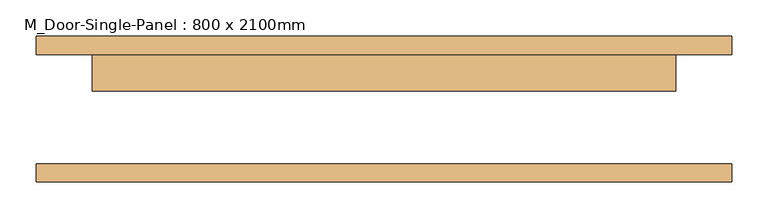
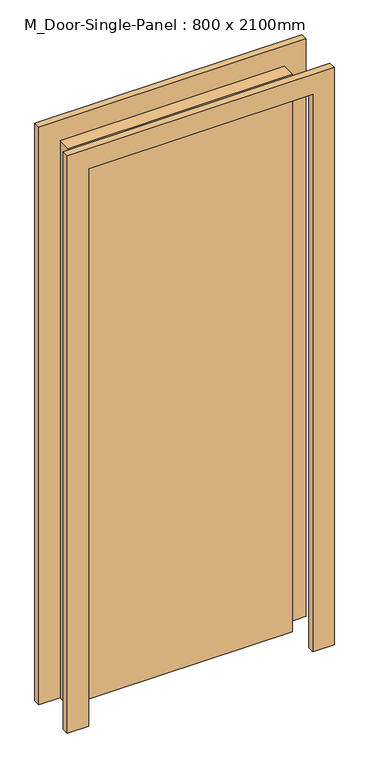
"""IFC4 building model written with IfcOpenShell, lengths in millimetres: door geometry, M_Door-Single-Panel : 800 x 2100mm."""

from ifc_helpers import new_model, si_unit, frame, origin, origin_with_axes, place, context, project, spatial, polyline, outline, extrude, source, transform, mapped, element, save


def m_door_single_panel_800_x_2100mm_d01656e8(model_context):
    return source(origin(), model_context, "Body", "SweptSolid", [
        extrude(outline(polyline([(400.0, 25.0), (-400.0, 25.0), (-400.0, 75.0), (400.0, 75.0), (400.0, 25.0)])), origin_with_axes(), (0.0, 0.0, 1.0), 2100.0),
        extrude(outline(polyline([(2176.2, 476.2), (2176.2, -476.2), (0.0, -476.2), (0.0, -400.0), (2100.0, -400.0), (2100.0, 400.0), (0.0, 400.0), (0.0, 476.2), (2176.2, 476.2)])), frame((0.0, -100.0, 0.0), z_axis=(0.0, 1.0, 0.0), x_axis=(0.0, 0.0, 1.0)), (0.0, 0.0, 1.0), 25.0),
        extrude(outline(polyline([(2176.2, -476.2), (0.0, -476.2), (0.0, -400.0), (2100.0, -400.0), (2100.0, 400.0), (0.0, 400.0), (0.0, 476.2), (2176.2, 476.2), (2176.2, -476.2)])), frame((0.0, 75.0, 0.0), z_axis=(0.0, 1.0, 0.0), x_axis=(0.0, 0.0, 1.0)), (0.0, 0.0, 1.0), 25.0),
    ])


if __name__ == "__main__":
    model = new_model("IFC4")
    model_context = context("Model", 3, world=origin())
    ifc_project = project(units=[si_unit("LENGTHUNIT", "METRE", prefix="MILLI")], contexts=[model_context])
    site = spatial("IfcSite", under=ifc_project)
    building = spatial("IfcBuilding", under=site)
    placement = place(None, origin())
    m_door_single_panel_800_x_2100mm_shape = m_door_single_panel_800_x_2100mm_d01656e8(model_context)
    element("IfcDoor", 1, ObjectType="M_Door-Single-Panel : 800 x 2100mm", at=placement, inside=building, context=model_context, shape_type="MappedRepresentation", body=[
        mapped(m_door_single_panel_800_x_2100mm_shape, transform((0.0, 0.0, 0.0), x_axis=(1.0, 0.0, 0.0), y_axis=(0.0, 1.0, 0.0), z_axis=(0.0, 0.0, 1.0))),
    ])
    save(model, "model.ifc")

# Revit data of these elements
# Type "M_Door-Single-Panel : 800 x 2100mm"
#   Type Mark = "41"
#   Construction Type Id = "DOOR"
#   Assembly Code = "C1020300"
#   Analytic Construction = "Wooden"
#   Thickness = 50 mm
#   Thermal Resistance (R) = 0.455703 (m²·K)/W
#   Swing Angle [instance default] = 90.00°
#   Heat Transfer Coefficient (U) = 2.19465 W/(m²·K)
#   Height = 2100 mm
#   Trim Projection Ext = 25 mm
#   Trim Projection Int = 25 mm
#   Trim Width = 80 mm
#   Width = 800 mm
#   Define Thermal Properties by = 1
#   Panel Material = Wood - Birch - Solid Stained Light Low Gloss
#   Trim Material = Paint - Sienna
#   Visual Light Transmittance = 0
#   Solar Heat Gain Coefficient = 0
#   Function = (empty or 0)
#   Wall Closure = (empty or 0)
# Element 1 (IfcDoor, "M_Door-Single-Panel : 800 x 2100mm")
#   Materials on its faces: "Paint - Sienna", "Wood - Birch - Solid Stained Light Low Gloss"
# Materials
#   "Wood - Birch - Solid Stained Light Low Gloss": class "Wood", colour RGB 210 159 95, transparency 0, Cost = 0
#   "Paint - Sienna": colour RGB 118 70 51, transparency 0, Cost = 0
